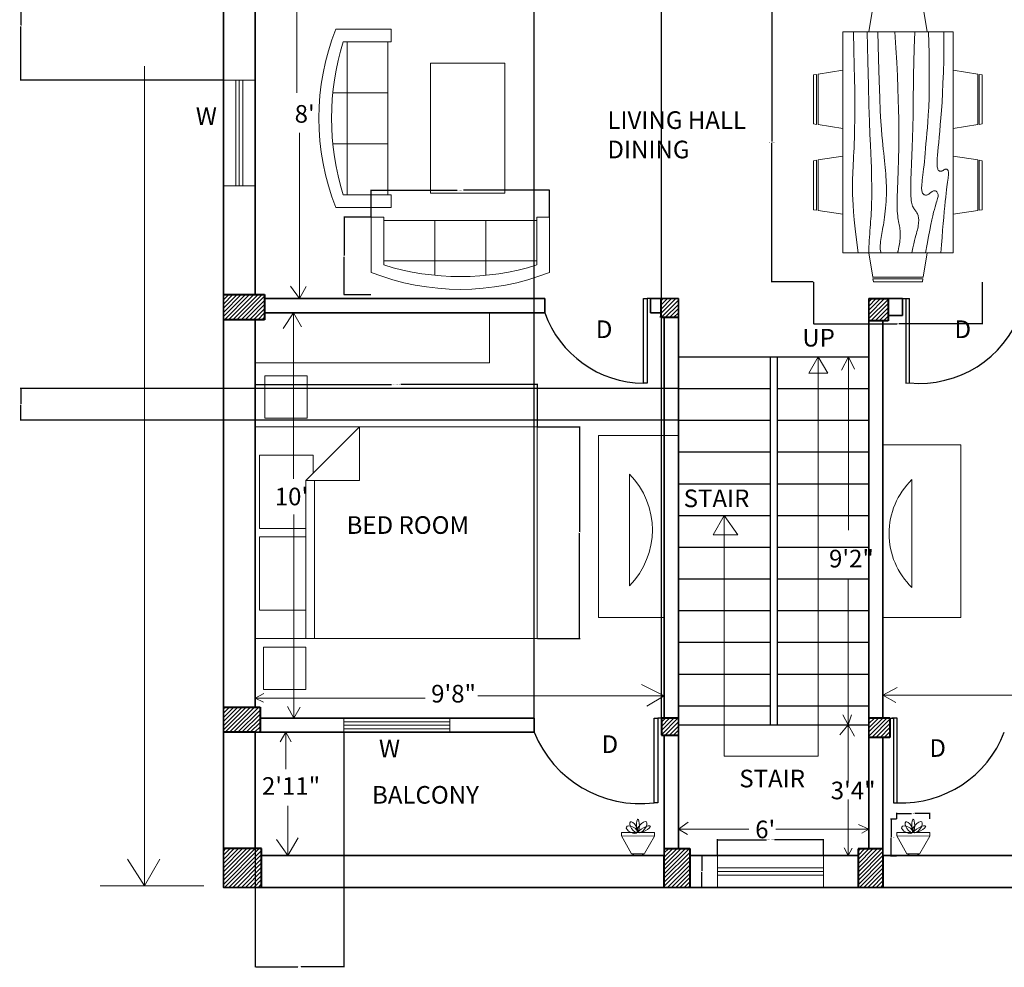
# Model space of a CAD drawing. Units: inches. Extents: x -34 to 385, y -422 to 64.
# Tile 1 of 3: x -34 to 246, y -422 to -153. Entities that reach past the tile are written whole.
import ezdxf

# ---------------------------------------------------------------- set-up
doc = ezdxf.new("R2010")
doc.units = ezdxf.units.IN
doc.header["$MEASUREMENT"] = 0
for name, color, linetype, lineweight in [('A-ANNO-DIMS', 2, 'Continuous', 13), ('A-ANNO-SYMB', 7, 'Continuous', 18), ('A-ANNO-TEXT', 7, 'Continuous', 18), ('A-AREA-IDEN', 7, 'Continuous', 25), ('A-COLS', 1, 'Continuous', 40), ('A-COLS-PATT', 252, 'Continuous', 13), ('A-DOOR', 3, 'Continuous', 25), ('A-FLOR-CASE', 32, 'Continuous', 20), ('A-FLOR-STRS', 7, 'Continuous', 25), ('A-FURN', 8, 'Continuous', 18), ('A-FURN-PLNT', 94, 'Continuous', 18), ('A-GLAZ', 4, 'Continuous', 18), ('A-WALL', 7, 'Continuous', 35)]:
    doc.layers.add(name, color=color, linetype=linetype, lineweight=lineweight)
doc.styles.get("Standard").update_dxf_attribs({"font": 'arial.ttf'})
doc.dimstyles.get("Standard").update_dxf_attribs({"dimtxt": 0.18, "dimasz": 0.18, "dimexe": 0.18, "dimexo": 0.0625, "dimgap": 0.09, "dimtad": 0, "dimtih": 1, "dimtoh": 1, "dimdec": 4, "dimzin": 0, "dimdsep": 46, "dimtxsty": 'Standard', "dimcen": 0.09, "dimadec": 0, "dimazin": 0, "dimtfac": 1, "dimtdec": 4, "dimtofl": 0, "dimtmove": 0, "dimatfit": 3, "dimfxl": 1, "dimtolj": 1, "dimtzin": 0, "dimarcsym": 0})

# ---------------------------------------------------------------- blocks, each defined once
blk = doc.blocks.new('Dining Set - 36 x 72 in.')
for p, q in [((-22.2343, 26.00059), (-23.4847, 17.99762)), ((-22.2304, 26), (-5.7608, 26)), ((-22, 27.5), (-22.1562, 26.50042)), ((-5.8416, 26.5), (-22.1534, 26.5)), ((-22, 27.5), (-6, 27.5)), ((-5.8437, 26.49966), (-6, 27.5)), ((-4.5152, 17.99762), (-5.7655, 25.99926)), ((5.7657, 26.00059), (4.5153, 17.99762)), ((5.7696, 26), (22.2392, 26)), ((6, 27.5), (5.8438, 26.50042)), ((22.1584, 26.5), (5.8466, 26.5)), ((6, 27.5), (22, 27.5)), ((22.1563, 26.49966), (22, 27.5)), ((23.4848, 17.99762), (22.2345, 25.99926)), ((36, 18), (-36, 18)), ((-36, 18), (-36, -18)), ((36, -18), (36, 18)), ((-45.5, 8), (-44.5004, 8.15617)), ((-45.5, 8), (-45.5, -8)), ((-44.5, -8.15843), (-44.5, 8.15338)), ((-44.0006, 8.23428), (-35.9976, 9.48474)), ((-44, 8.23041), (-44, -8.23915)), ((44.0006, 8.23428), (35.9976, 9.48474)), ((44, 8.23041), (44, -8.23915)), ((44.5, -8.15843), (44.5, 8.15338)), ((45.5, 8), (44.5005, 8.15617)), ((45.5, 8), (45.5, -8)), ((-44.4997, -8.15631), (-45.5, -8)), ((-35.9976, -9.48476), (-43.9993, -8.2345)), ((35.9976, -9.48476), (43.9993, -8.2345)), ((44.4997, -8.15631), (45.5, -8)), ((-36, -18), (36, -18)), ((-22.2343, -26.0006), (-23.4847, -17.99762)), ((-4.5152, -17.99762), (-5.7655, -25.99928)), ((5.7657, -26.0006), (4.5153, -17.99762)), ((23.4848, -17.99762), (22.2345, -25.99928)), ((-22.2304, -26), (-5.7608, -26)), ((-22, -27.5), (-22.1562, -26.50044)), ((-5.8416, -26.5), (-22.1534, -26.5)), ((-22, -27.5), (-6, -27.5)), ((-5.8437, -26.49967), (-6, -27.5)), ((5.7696, -26), (22.2392, -26)), ((6, -27.5), (5.8438, -26.50044)), ((22.1584, -26.5), (5.8466, -26.5)), ((6, -27.5), (22, -27.5)), ((22.1563, -26.49967), (22, -27.5))]:
    blk.add_line(p, q)
for points in [[(-36, 15), (-31.1772, 14.97754), (-26.8079, 14.91406), (-22.8538, 14.81543), (-19.276, 14.6875), (-16.0362, 14.53613), (-13.0957, 14.36718), (-10.4159, 14.18652), (-7.9583, 14), (-5.6904, 13.81315), (-3.6035, 13.63021), (-1.6954, 13.45508), (0.0365, 13.29166), (1.5945, 13.14388), (2.9811, 13.01562), (4.1988, 12.9108), (5.25, 12.83333), (6.1393, 12.78613), (6.8802, 12.76823), (7.4883, 12.77767), (7.9792, 12.8125), (8.3685, 12.87077), (8.6719, 12.95052), (8.9049, 13.0498), (9.0833, 13.16666), (9.2205, 13.29899), (9.3216, 13.44401), (9.3895, 13.59879), (9.4271, 13.76041), (9.4373, 13.92594), (9.4232, 14.09245), (9.3875, 14.257), (9.3333, 14.41666), (9.2638, 14.56917), (9.1836, 14.71484), (9.0975, 14.85465), (9.0104, 14.98958), (8.9272, 15.1206), (8.8529, 15.2487), (8.7922, 15.37483), (8.75, 15.5), (8.7305, 15.62467), (8.7344, 15.74739), (8.7617, 15.86621), (8.8125, 15.97916), (8.8867, 16.08431), (8.9844, 16.17968), (9.1055, 16.26334), (9.25, 16.33333), (9.4189, 16.38802), (9.6172, 16.42708), (9.8506, 16.45052), (10.125, 16.45833), (10.4463, 16.45052), (10.8203, 16.42708), (11.2529, 16.38802), (11.75, 16.33333), (12.3184, 16.26318), (12.9694, 16.17838), (13.7151, 16.07991), (14.5677, 15.96875), (15.5395, 15.84586), (16.6426, 15.71224), (17.8893, 15.56884), (19.2917, 15.41666), (20.859, 15.25667), (22.5879, 15.08984), (24.4721, 14.91715), (26.5052, 14.73958), (28.6809, 14.5581), (30.9929, 14.3737), (33.4347, 14.18733), (36, 14)], [(-36, 10), (-28.9766, 10.14274), (-23.1725, 10.20442), (-18.4241, 10.19775), (-14.5677, 10.13541), (-11.4399, 10.03011), (-8.877, 9.89453), (-6.7154, 9.74137), (-4.7917, 9.58333), (-2.9698, 9.43082), (-1.2246, 9.28515), (0.4415, 9.14534), (2.026, 9.01041), (3.5266, 8.87939), (4.9408, 8.7513), (6.266, 8.62516), (7.5, 8.5), (8.6411, 8.37549), (9.6914, 8.2539), (10.6538, 8.13818), (11.5312, 8.03125), (12.3267, 7.93603), (13.043, 7.85547), (13.6831, 7.79248), (14.25, 7.75), (14.7471, 7.7303), (15.1797, 7.73307), (15.5537, 7.75732), (15.875, 7.80208), (16.1494, 7.86637), (16.3828, 7.94922), (16.5811, 8.04964), (16.75, 8.16666), (16.8944, 8.29915), (17.0143, 8.44531), (17.1089, 8.60319), (17.1771, 8.77083), (17.218, 8.94629), (17.2305, 9.1276), (17.2137, 9.31282), (17.1667, 9.5), (17.0895, 9.6875), (16.987, 9.875), (16.8649, 10.0625), (16.7292, 10.25), (16.5856, 10.4375), (16.4401, 10.625), (16.2985, 10.8125), (16.1667, 11), (16.05, 11.18733), (15.9518, 11.3737), (15.8752, 11.5581), (15.8229, 11.73958), (15.798, 11.91715), (15.8034, 12.08984), (15.842, 12.25667), (15.9167, 12.41666), (16.0295, 12.56836), (16.1784, 12.70833), (16.3605, 12.83268), (16.5729, 12.9375), (16.8127, 13.01888), (17.0768, 13.07291), (17.3625, 13.0957), (17.6667, 13.08333), (17.9894, 13.03312), (18.3418, 12.94726), (18.7382, 12.82918), (19.1927, 12.68229), (19.7195, 12.51001), (20.3327, 12.31575), (21.0465, 12.10294), (21.875, 11.875), (22.8357, 11.63354), (23.959, 11.37304), (25.2786, 11.08618), (26.8282, 10.76562), (28.6414, 10.40405), (30.752, 9.99414), (33.1936, 9.52856), (36, 9)], [(-36, 5.5), (-30.7157, 5.3348), (-26.069, 5.20963), (-21.9946, 5.11767), (-18.4271, 5.05208), (-15.3009, 5.00602), (-12.5508, 4.97265), (-10.1112, 4.94515), (-7.9167, 4.91666), (-5.909, 4.88167), (-4.0586, 4.83984), (-2.3429, 4.79215), (-0.7396, 4.73958), (0.7739, 4.6831), (2.22, 4.6237), (3.6213, 4.56233), (5, 4.5), (6.373, 4.43782), (7.7344, 4.3776), (9.0723, 4.32129), (10.375, 4.27083), (11.6309, 4.22819), (12.8281, 4.19531), (13.9551, 4.17415), (15, 4.16666), (15.954, 4.17448), (16.819, 4.19791), (17.6001, 4.23698), (18.3021, 4.29166), (18.9299, 4.36198), (19.4883, 4.44791), (19.9823, 4.54948), (20.4167, 4.66666), (20.7969, 4.79899), (21.1302, 4.94401), (21.4245, 5.09879), (21.6875, 5.26041), (21.9271, 5.42594), (22.1511, 5.59245), (22.3672, 5.757), (22.5834, 5.91666), (22.8065, 6.06868), (23.0404, 6.21093), (23.2879, 6.34147), (23.5521, 6.45833), (23.8358, 6.55957), (24.142, 6.64323), (24.4735, 6.70735), (24.8334, 6.75), (25.2235, 6.76969), (25.642, 6.76692), (26.0858, 6.74267), (26.5521, 6.69791), (27.0379, 6.63362), (27.5404, 6.55078), (28.0565, 6.45036), (28.5834, 6.33333), (29.1242, 6.19987), (29.7071, 6.04687), (30.3661, 5.87044), (31.1354, 5.66666), (32.0493, 5.43164), (33.142, 5.16146), (34.4475, 4.85221), (36, 4.5)], [(-36, -1), (-30.7915, -0.6591), (-26.0195, -0.38216), (-21.6519, -0.16284), (-17.6563, 0.00521), (-14.0005, 0.12833), (-10.6523, 0.21289), (-7.5796, 0.26522), (-4.75, 0.29166), (-2.134, 0.29793), (0.2878, 0.28711), (2.5317, 0.26163), (4.6146, 0.22396), (6.5529, 0.17651), (8.3633, 0.12174), (10.0623, 0.06209), (11.6667, 0), (13.1899, -0.06201), (14.6341, -0.1211), (15.9982, -0.17432), (17.2813, -0.21875), (18.4823, -0.25147), (19.6003, -0.26953), (20.6343, -0.27002), (21.5834, -0.25), (22.4481, -0.20768), (23.2357, -0.14584), (23.9549, -0.06836), (24.6146, 0.02083), (25.2235, 0.11784), (25.7904, 0.21875), (26.3241, 0.31966), (26.8334, 0.41666), (27.3265, 0.50618), (27.8099, 0.58593), (28.2894, 0.65397), (28.7709, 0.70833), (29.2601, 0.74707), (29.763, 0.76823), (30.2855, 0.76985), (30.8334, 0.75), (31.4088, 0.70784), (31.9994, 0.64713), (32.589, 0.57275), (33.1615, 0.48958), (33.7008, 0.4025), (34.1908, 0.3164), (34.6153, 0.23616), (34.9584, 0.16666), (35.2099, 0.11165), (35.3848, 0.07031), (35.504, 0.04069), (35.5886, 0.02083), (35.6594, 0.00879), (35.7377, 0.0026), (35.8442, 0.00032), (36, 0)], [(-36, -6.5), (-27.1843, -6.31267), (-20.084, -6.1263), (-14.469, -5.9419), (-10.1094, -5.76042), (-6.7752, -5.58285), (-4.2363, -5.41016), (-2.2629, -5.24333), (-0.625, -5.08334), (0.8708, -4.93099), (2.2715, -4.78646), (3.5872, -4.64974), (4.8281, -4.52084), (6.0046, -4.39974), (7.127, -4.28646), (8.2053, -4.18099), (9.25, -4.08334), (10.2705, -3.99382), (11.2734, -3.91407), (12.2647, -3.84603), (13.25, -3.79167), (14.2354, -3.75293), (15.2266, -3.73177), (16.2295, -3.73015), (17.25, -3.75), (18.2912, -3.79248), (19.3451, -3.85547), (20.4009, -3.93604), (21.4479, -4.03125), (22.4754, -4.13819), (23.4727, -4.25391), (24.4289, -4.37549), (25.3334, -4.5), (26.1785, -4.62492), (26.9694, -4.74935), (27.7145, -4.87281), (28.4219, -4.99479), (29.1, -5.11483), (29.7572, -5.23242), (30.4016, -5.34709), (31.0417, -5.45834), (31.6837, -5.56437), (32.3262, -5.65821), (32.9658, -5.73153), (33.599, -5.77604), (34.2224, -5.78345), (34.8327, -5.74545), (35.4264, -5.65373), (36, -5.5)], [(-36, -10), (-26.4022, -9.81299), (-18.4675, -9.62891), (-11.9839, -9.45069), (-6.7396, -9.28125), (-2.5226, -9.12354), (0.8789, -8.98047), (3.6769, -8.85498), (6.0833, -8.75), (8.2767, -8.66765), (10.3021, -8.60677), (12.1712, -8.56543), (13.8958, -8.54167), (15.4876, -8.53353), (16.9583, -8.53907), (18.3197, -8.55632), (19.5834, -8.58334), (20.7616, -8.61841), (21.8685, -8.66081), (22.9188, -8.71004), (23.9271, -8.76563), (24.9081, -8.82707), (25.8763, -8.89388), (26.8465, -8.96558), (27.8334, -9.04167), (28.8474, -9.12118), (29.8828, -9.20117), (30.93, -9.27824), (31.9792, -9.34896), (33.0205, -9.40991), (34.0443, -9.45768), (35.0407, -9.48885), (36, -9.5)], [(-36, -14.5), (-30.0881, -14.33513), (-25.0332, -14.21224), (-20.7312, -14.12647), (-17.0781, -14.07292), (-13.97, -14.04671), (-11.3027, -14.04297), (-8.9724, -14.05681), (-6.875, -14.08334), (-4.9224, -14.11833), (-3.0905, -14.16016), (-1.3709, -14.20785), (0.2448, -14.26042), (1.7647, -14.3169), (3.1973, -14.3763), (4.5507, -14.43767), (5.8333, -14.5), (7.0554, -14.5621), (8.235, -14.62175), (9.3922, -14.67652), (10.5469, -14.72396), (11.7192, -14.76164), (12.929, -14.78711), (14.1965, -14.79794), (15.5417, -14.79167), (16.9933, -14.76424), (18.6152, -14.70508), (20.4804, -14.60197), (22.6615, -14.44271), (25.2312, -14.21509), (28.2624, -13.9069), (31.8277, -13.50594), (36, -13)]]:
    blk.add_lwpolyline(points)
blk = doc.blocks.new('Sofa - Roundback 7 ft.')
for p, q in [((-12.00002, -32.4421), (-12.00003, -6.5971)), ((11.99997, -32.4421), (11.99998, -6.5971)), ((-36.000027, -34), (-36.000027, -11.4696)), ((-35.999844, -13.3819), (35.9998, -13.3819)), ((35.99998, -34), (35.99998, -11.4696)), ((-36.000027, -32.4421), (35.99998, -32.4421))]:
    blk.add_line(p, q)
for points in [[(-36.000027, -34), (-42.000027, -34), (-42.000027, -8)], [(41.99998, -8), (41.99998, -34), (35.99998, -34)]]:
    blk.add_lwpolyline(points)
for centre, radius, start, end in [((0, -114.25), 114.25, 68.43141, 111.5686), ((-0.00001, -127.1968), 121.1968, 72.72033, 107.2797)]:
    blk.add_arc(centre, radius, start, end)
blk = doc.blocks.new('Bed - Queen')
for p, q in [((0, -80.00003), (0, 0)), ((0, 0), (59.99999, 0)), ((59.99999, 0), (59.99999, -80.00003)), ((7.99999, -1.2), (28.79998, -1.2)), ((7.99999, -14.4), (7.99999, -1.2)), ((28.79998, -1.2), (28.79998, -14.4)), ((31.19999, -1.2), (51.99999, -1.2)), ((31.19999, -14.4), (31.19999, -1.2)), ((51.99999, -1.2), (51.99999, -16.4)), ((0, -14.4), (44.8, -14.4)), ((59.99999, -29.6), (44.8, -14.4)), ((44.8, -14.4), (44.8, -29.6)), ((51.99999, -16.4), (46.79936, -16.4)), ((44.8, -16.8), (0, -16.8)), ((44.8, -29.6), (59.99999, -29.6)), ((59.99999, -80.00003), (0, -80.00003))]:
    blk.add_line(p, q)
blk = doc.blocks.new('WIN-30IN-9IN-WALL')
for p, q in [((0, 9), (0, 0)), ((30, 9), (30, 0)), ((0, 5.5), (30, 5.5)), ((0, 4.5), (30, 4.5)), ((0, 3.5), (30, 3.5))]:
    blk.add_line(p, q)
blk = doc.blocks.new('WIN-30IN-4IN-WALL')
for p, q in [((0, 4), (0, 0)), ((0, 3), (30, 3)), ((30, 4), (30, 0)), ((0, 2), (30, 2)), ((0, 1), (30, 1))]:
    blk.add_line(p, q)
blk = doc.blocks.new('DOOR-LEAF-24IN')
for p, q in [((1, 24), (0, 24)), ((0, 24), (0, 0)), ((1, 0), (1, 24)), ((0, 0), (1, 0)), ((2, 0), (1, 0))]:
    blk.add_line(p, q)
blk = doc.blocks.new('NIGHTSTAND-12IN')
blk.add_lwpolyline([(12, 0), (0, 0), (0, 12), (12, 12)], close=True)
blk = doc.blocks.new('BALCONY-PLANTER')
for p, q in [((0, 5.57), (0, 6.56)), ((0, 6.56), (9.42, 6.56)), ((9.42, 6.56), (9.42, 5.54)), ((2.92, 0.52), (0, 5.57)), ((0, 5.57), (9.42, 5.54)), ((9.42, 5.54), (6.54, 0.56))]:
    blk.add_line(p, q)
blk.add_arc((4.7, 3.31), 3.31, 237.326, 303.729)
for centre, major_axis, ratio in [((2.96, 7.36), (1.54, -0.75), 0.479353), ((3.53, 8.09), (0.98, -1.48), 0.414718), ((4.71, 8.47), (0, -1.91), 0.211909), ((5.9, 8.07), (-1.19, -1.51), 0.459362), ((6.52, 7.49), (-1.74, -0.91), 0.246731)]:
    blk.add_ellipse(centre, major_axis=major_axis, ratio=ratio)
blk = doc.blocks.new('*D14')
at = {"layer": 'A-ANNO-DIMS', "color": 0, "lineweight": -2, "transparency": 16777216}
for p, q in [((164.36, -390.08), (164.36, -385.46)), ((164.54, -385.64), (178.24, -385.64)), ((194.18, -385.64), (180.48, -385.64)), ((194.36, -390.08), (194.36, -385.46))]:
    blk.add_line(p, q, dxfattribs=at)
at = {"layer": 'A-ANNO-DIMS', "color": 0, "transparency": 16777216}
for points in [[(164.54, -385.61), (164.54, -385.67), (164.36, -385.64)], [(194.18, -385.61), (194.18, -385.67), (194.36, -385.64)]]:
    blk.add_solid(points, dxfattribs=at)
at = {"layer": 'Defpoints', "color": 0, "transparency": 16777216}
for p in [(194.36, -385.64), (164.36, -390.14), (194.36, -390.14)]:
    blk.add_point(p, dxfattribs=at)
at = {"layer": 'A-ANNO-DIMS', "color": 0, "transparency": 16777216, "insert": (179.36, -385.64), "char_height": 0.18, "attachment_point": 5}
blk.add_mtext('\\A1;WINDOW 30 TYP.', dxfattribs=at)
blk = doc.blocks.new('*D15')
at = {"layer": 'A-ANNO-DIMS', "color": 0, "lineweight": -2, "transparency": 16777216}
for p, q in [((164.3, -390.14), (159.68, -390.14)), ((159.86, -390.32), (159.86, -394.46)), ((159.86, -398.96), (159.86, -394.82)), ((164.3, -399.14), (159.68, -399.14))]:
    blk.add_line(p, q, dxfattribs=at)
at = {"layer": 'A-ANNO-DIMS', "color": 0, "transparency": 16777216}
for points in [[(159.83, -390.32), (159.89, -390.32), (159.86, -390.14)], [(159.83, -398.96), (159.89, -398.96), (159.86, -399.14)]]:
    blk.add_solid(points, dxfattribs=at)
at = {"layer": 'Defpoints', "color": 0, "transparency": 16777216}
for p in [(159.86, -390.14), (164.36, -390.14), (164.36, -399.14)]:
    blk.add_point(p, dxfattribs=at)
at = {"layer": 'A-ANNO-DIMS', "color": 0, "transparency": 16777216, "insert": (159.86, -394.64), "char_height": 0.18, "attachment_point": 5}
blk.add_mtext('\\A1;9 TYP.', dxfattribs=at)
blk = doc.blocks.new('*D20')
at = {"layer": 'A-ANNO-DIMS', "color": 0, "lineweight": -2, "transparency": 16777216}
for p, q in [((33.26, -268.45), (33.26, -256.33)), ((33.44, -256.51), (71.95, -256.51)), ((113.08, -256.51), (74.56, -256.51)), ((113.26, -268.45), (113.26, -256.33))]:
    blk.add_line(p, q, dxfattribs=at)
at = {"layer": 'A-ANNO-DIMS', "color": 0, "transparency": 16777216}
for points in [[(33.44, -256.48), (33.44, -256.54), (33.26, -256.51)], [(113.08, -256.48), (113.08, -256.54), (113.26, -256.51)]]:
    blk.add_solid(points, dxfattribs=at)
at = {"layer": 'Defpoints', "color": 0, "transparency": 16777216}
for p in [(33.26, -256.51), (33.26, -268.51), (113.26, -268.51)]:
    blk.add_point(p, dxfattribs=at)
at = {"layer": 'A-ANNO-DIMS', "color": 0, "transparency": 16777216, "insert": (73.26, -256.51), "char_height": 0.18, "attachment_point": 5}
blk.add_mtext('\\A1;QUEEN BED 80 TYP.', dxfattribs=at)
blk = doc.blocks.new('*D21')
at = {"layer": 'A-ANNO-DIMS', "color": 0, "lineweight": -2, "transparency": 16777216}
for p, q in [((113.32, -268.51), (125.44, -268.51)), ((125.26, -268.69), (125.26, -298.33)), ((125.26, -328.33), (125.26, -298.7)), ((113.32, -328.51), (125.44, -328.51))]:
    blk.add_line(p, q, dxfattribs=at)
at = {"layer": 'A-ANNO-DIMS', "color": 0, "transparency": 16777216}
for points in [[(125.23, -268.69), (125.29, -268.69), (125.26, -268.51)], [(125.23, -328.33), (125.29, -328.33), (125.26, -328.51)]]:
    blk.add_solid(points, dxfattribs=at)
at = {"layer": 'Defpoints', "color": 0, "transparency": 16777216}
for p in [(113.26, -268.51), (125.26, -268.51), (113.26, -328.51)]:
    blk.add_point(p, dxfattribs=at)
at = {"layer": 'A-ANNO-DIMS', "color": 0, "transparency": 16777216, "insert": (125.26, -298.51), "char_height": 0.18, "attachment_point": 5}
blk.add_mtext('\\A1;60 TYP.', dxfattribs=at)
blk = doc.blocks.new('*D22')
at = {"layer": 'A-ANNO-DIMS', "color": 0, "lineweight": -2, "transparency": 16777216}
for p, q in [((66.13, -208.95), (66.13, -201.24)), ((66.31, -201.42), (90.53, -201.42)), ((116.57, -201.42), (92.34, -201.42)), ((116.75, -208.95), (116.75, -201.24))]:
    blk.add_line(p, q, dxfattribs=at)
at = {"layer": 'A-ANNO-DIMS', "color": 0, "transparency": 16777216}
for points in [[(66.31, -201.39), (66.31, -201.45), (66.13, -201.42)], [(116.57, -201.39), (116.57, -201.45), (116.75, -201.42)]]:
    blk.add_solid(points, dxfattribs=at)
at = {"layer": 'Defpoints', "color": 0, "transparency": 16777216}
for p in [(66.13, -201.42), (66.13, -209.01), (116.75, -209.01)]:
    blk.add_point(p, dxfattribs=at)
at = {"layer": 'A-ANNO-DIMS', "color": 0, "transparency": 16777216, "insert": (91.44, -201.42), "char_height": 0.18, "attachment_point": 5}
blk.add_mtext('\\A1;SOFA 51 TYP.', dxfattribs=at)
blk = doc.blocks.new('*D23')
at = {"layer": 'A-ANNO-DIMS', "color": 0, "lineweight": -2, "transparency": 16777216}
for p, q in [((66.06, -209.01), (58.35, -209.01)), ((58.53, -209.19), (58.53, -219.88)), ((58.53, -230.93), (58.53, -220.24)), ((66.06, -231.11), (58.35, -231.11))]:
    blk.add_line(p, q, dxfattribs=at)
at = {"layer": 'A-ANNO-DIMS', "color": 0, "transparency": 16777216}
for points in [[(58.5, -209.19), (58.56, -209.19), (58.53, -209.01)], [(58.5, -230.93), (58.56, -230.93), (58.53, -231.11)]]:
    blk.add_solid(points, dxfattribs=at)
at = {"layer": 'Defpoints', "color": 0, "transparency": 16777216}
for p in [(66.13, -209.01), (58.53, -231.11), (66.13, -231.11)]:
    blk.add_point(p, dxfattribs=at)
at = {"layer": 'A-ANNO-DIMS', "color": 0, "transparency": 16777216, "insert": (58.53, -220.06), "char_height": 0.18, "attachment_point": 5}
blk.add_mtext('\\A1;22 TYP.', dxfattribs=at)
blk = doc.blocks.new('*D26')
at = {"layer": 'A-ANNO-DIMS', "color": 0, "lineweight": -2, "transparency": 16777216}
for p, q in [((215.08, -379.77), (213.38, -379.77)), ((213.56, -379.95), (213.56, -384.87)), ((213.56, -390.15), (213.56, -385.23)), ((215.08, -390.33), (213.38, -390.33))]:
    blk.add_line(p, q, dxfattribs=at)
at = {"layer": 'A-ANNO-DIMS', "color": 0, "transparency": 16777216}
for points in [[(213.53, -379.95), (213.59, -379.95), (213.56, -379.77)], [(213.53, -390.15), (213.59, -390.15), (213.56, -390.33)]]:
    blk.add_solid(points, dxfattribs=at)
at = {"layer": 'Defpoints', "color": 0, "transparency": 16777216}
for p in [(213.56, -379.77), (215.14, -379.77), (215.14, -390.33)]:
    blk.add_point(p, dxfattribs=at)
at = {"layer": 'A-ANNO-DIMS', "color": 0, "transparency": 16777216, "insert": (213.56, -385.05), "char_height": 0.18, "attachment_point": 5}
blk.add_mtext('\\A1;PLANTER 11 TYP.', dxfattribs=at)
blk = doc.blocks.new('*D27')
at = {"layer": 'A-ANNO-DIMS', "color": 0, "lineweight": -2, "transparency": 16777216}
for p, q in [((215.14, -379.7), (215.14, -378)), ((215.32, -378.18), (219.39, -378.18)), ((224.38, -378.18), (220.31, -378.18)), ((224.56, -379.7), (224.56, -378))]:
    blk.add_line(p, q, dxfattribs=at)
at = {"layer": 'A-ANNO-DIMS', "color": 0, "transparency": 16777216}
for points in [[(215.32, -378.15), (215.32, -378.21), (215.14, -378.18)], [(224.38, -378.15), (224.38, -378.21), (224.56, -378.18)]]:
    blk.add_solid(points, dxfattribs=at)
at = {"layer": 'Defpoints', "color": 0, "transparency": 16777216}
for p in [(224.56, -378.18), (215.14, -379.77), (224.56, -379.77)]:
    blk.add_point(p, dxfattribs=at)
at = {"layer": 'A-ANNO-DIMS', "color": 0, "transparency": 16777216, "insert": (219.85, -378.18), "char_height": 0.18, "attachment_point": 5}
blk.add_mtext('\\A1;9 TYP.', dxfattribs=at)
blk = doc.blocks.new('*D32')
at = {"layer": 'A-ANNO-DIMS', "color": 0, "lineweight": -2, "transparency": 16777216}
for p, q in [((191.51, -148.21), (179.52, -148.21)), ((179.7, -148.39), (179.7, -187.61)), ((179.7, -227.2), (179.7, -187.98)), ((191.51, -227.38), (179.52, -227.38))]:
    blk.add_line(p, q, dxfattribs=at)
at = {"layer": 'A-ANNO-DIMS', "color": 0, "transparency": 16777216}
for points in [[(179.67, -148.39), (179.73, -148.39), (179.7, -148.21)], [(179.67, -227.2), (179.73, -227.2), (179.7, -227.38)]]:
    blk.add_solid(points, dxfattribs=at)
at = {"layer": 'Defpoints', "color": 0, "transparency": 16777216}
for p in [(191.58, -148.21), (179.7, -227.38), (191.58, -227.38)]:
    blk.add_point(p, dxfattribs=at)
at = {"layer": 'A-ANNO-DIMS', "color": 0, "transparency": 16777216, "insert": (179.7, -187.79), "char_height": 0.18, "attachment_point": 5}
blk.add_mtext('\\A1;DINING SET 79', dxfattribs=at)
blk = doc.blocks.new('*D33')
at = {"layer": 'A-ANNO-DIMS', "color": 0, "lineweight": -2, "transparency": 16777216}
for p, q in [((191.58, -227.44), (191.58, -239.43)), ((239.42, -227.44), (239.42, -239.43)), ((191.76, -239.25), (215.28, -239.25)), ((239.24, -239.25), (215.72, -239.25))]:
    blk.add_line(p, q, dxfattribs=at)
at = {"layer": 'A-ANNO-DIMS', "color": 0, "transparency": 16777216}
for points in [[(191.76, -239.22), (191.76, -239.28), (191.58, -239.25)], [(239.24, -239.22), (239.24, -239.28), (239.42, -239.25)]]:
    blk.add_solid(points, dxfattribs=at)
at = {"layer": 'Defpoints', "color": 0, "transparency": 16777216}
for p in [(191.58, -227.38), (239.42, -227.38), (239.42, -239.25)]:
    blk.add_point(p, dxfattribs=at)
at = {"layer": 'A-ANNO-DIMS', "color": 0, "transparency": 16777216, "insert": (215.5, -239.25), "char_height": 0.18, "attachment_point": 5}
blk.add_mtext('\\A1;48', dxfattribs=at)
blk = doc.blocks.new('*D36')
at = {"layer": 'A-ANNO-DIMS', "color": 0, "lineweight": -2, "transparency": 16777216}
for p, q in [((24.19, -139.38), (-33.38, -139.38)), ((-33.2, -139.56), (-33.2, -154.58)), ((-33.2, -169.95), (-33.2, -154.94)), ((24.19, -170.13), (-33.38, -170.13))]:
    blk.add_line(p, q, dxfattribs=at)
at = {"layer": 'A-ANNO-DIMS', "color": 0, "transparency": 16777216}
for points in [[(-33.23, -139.56), (-33.17, -139.56), (-33.2, -139.38)], [(-33.23, -169.95), (-33.17, -169.95), (-33.2, -170.13)]]:
    blk.add_solid(points, dxfattribs=at)
at = {"layer": 'Defpoints', "color": 0, "transparency": 16777216}
for p in [(24.26, -139.38), (-33.2, -170.13), (24.26, -170.13)]:
    blk.add_point(p, dxfattribs=at)
at = {"layer": 'A-ANNO-DIMS', "color": 0, "transparency": 16777216, "insert": (-33.2, -154.76), "char_height": 0.18, "attachment_point": 5}
blk.add_mtext('\\A1;30.75', dxfattribs=at)
blk = doc.blocks.new('*D38')
at = {"layer": 'A-ANNO-DIMS', "color": 0, "lineweight": -2, "transparency": 16777216}
for p, q in [((153.19, -257.63), (-33.38, -257.63)), ((-33.2, -257.81), (-33.2, -261.95)), ((-33.2, -266.45), (-33.2, -262.31)), ((153.19, -266.63), (-33.38, -266.63))]:
    blk.add_line(p, q, dxfattribs=at)
at = {"layer": 'A-ANNO-DIMS', "color": 0, "transparency": 16777216}
for points in [[(-33.23, -257.81), (-33.17, -257.81), (-33.2, -257.63)], [(-33.23, -266.45), (-33.17, -266.45), (-33.2, -266.63)]]:
    blk.add_solid(points, dxfattribs=at)
at = {"layer": 'Defpoints', "color": 0, "transparency": 16777216}
for p in [(153.26, -257.63), (-33.2, -266.63), (153.26, -266.63)]:
    blk.add_point(p, dxfattribs=at)
at = {"layer": 'A-ANNO-DIMS', "color": 0, "transparency": 16777216, "insert": (-33.2, -262.13), "char_height": 0.18, "attachment_point": 5}
blk.add_mtext('\\A1;9', dxfattribs=at)
blk = doc.blocks.new('*D39')
at = {"layer": 'A-ANNO-DIMS', "color": 0, "lineweight": -2, "transparency": 16777216}
for p, q in [((112.34, -351.08), (112.34, 63.89)), ((112.52, 63.71), (129.99, 63.71)), ((148.25, 63.71), (130.78, 63.71)), ((148.43, -351.08), (148.43, 63.89))]:
    blk.add_line(p, q, dxfattribs=at)
at = {"layer": 'A-ANNO-DIMS', "color": 0, "transparency": 16777216}
for points in [[(112.52, 63.74), (112.52, 63.68), (112.34, 63.71)], [(148.25, 63.74), (148.25, 63.68), (148.43, 63.71)]]:
    blk.add_solid(points, dxfattribs=at)
at = {"layer": 'Defpoints', "color": 0, "transparency": 16777216}
for p in [(148.43, 63.71), (112.34, -351.14), (148.43, -351.14)]:
    blk.add_point(p, dxfattribs=at)
at = {"layer": 'A-ANNO-DIMS', "color": 0, "transparency": 16777216, "insert": (130.38, 63.71), "char_height": 0.18, "attachment_point": 5}
blk.add_mtext('\\A1;36.09', dxfattribs=at)
blk = doc.blocks.new('*D40')
at = {"layer": 'A-ANNO-DIMS', "color": 0, "lineweight": -2, "transparency": 16777216}
for p, q in [((33.26, -355.21), (33.26, -421.82)), ((58.42, -355.21), (58.42, -421.82)), ((33.44, -421.64), (45.37, -421.64)), ((58.24, -421.64), (46.3, -421.64))]:
    blk.add_line(p, q, dxfattribs=at)
at = {"layer": 'A-ANNO-DIMS', "color": 0, "transparency": 16777216}
for points in [[(33.44, -421.61), (33.44, -421.67), (33.26, -421.64)], [(58.24, -421.61), (58.24, -421.67), (58.42, -421.64)]]:
    blk.add_solid(points, dxfattribs=at)
at = {"layer": 'Defpoints', "color": 0, "transparency": 16777216}
for p in [(33.26, -355.14), (58.42, -355.14), (58.42, -421.64)]:
    blk.add_point(p, dxfattribs=at)
at = {"layer": 'A-ANNO-DIMS', "color": 0, "transparency": 16777216, "insert": (45.84, -421.64), "char_height": 0.18, "attachment_point": 5}
blk.add_mtext('\\A1;25.166', dxfattribs=at)

msp = doc.modelspace()

# ---------------------------------------------------------------- hatches: boundary and pattern name
at = {"layer": 'A-COLS-PATT'}
h = msp.add_hatch(dxfattribs=at)
h.set_pattern_fill('ANSI31', color=256, scale=6.7)
h.set_pattern_definition([(45, (-1587.6103, -800.894), (-0.59220193, 0.59220193), [])])
h.paths.add_polyline_path([(34.5325, 20.857), (24.2567, 20.857), (24.2567, 10.5552), (34.5325, 10.5552)])
h.paths.add_polyline_path([(155.6882, 20.857), (147.6505, 20.857), (147.6505, 8.8355), (155.6882, 8.8355)])
h.paths.add_polyline_path([(214.1102, 20.857), (204.3358, 20.857), (204.3358, 9.8804), (214.1102, 9.8804)])
h.paths.add_polyline_path([(336.2567, 20.857), (324.9664, 20.857), (324.9664, 9.4113), (336.2567, 9.4113)])
h.paths.add_polyline_path([(336.2567, -129.6656), (324.4892, -129.6656), (324.4892, -138.8931), (336.2567, -138.8931)])
h.paths.add_polyline_path([(212.9763, -130.7216), (204.8831, -130.7216), (204.8831, -136.143), (212.9763, -136.143)])
h.paths.add_polyline_path([(154.6774, -130.7571), (147.9004, -130.7571), (147.9004, -136.143), (154.6774, -136.143)])
h.paths.add_polyline_path([(36.3503, -129.7825), (24.2567, -129.7825), (24.2567, -139.3836), (36.3503, -139.3836)])
h.paths.add_polyline_path([(35.9496, -230.9729), (24.2567, -230.9729), (24.2567, -238.1404), (35.9496, -238.1404)])
h.paths.add_polyline_path([(153.2567, -232.143), (148.2796, -232.143), (148.2796, -237.1221), (148.2796, -237.5145), (153.2567, -237.5145)])
h.paths.add_polyline_path([(212.7, -232.143), (207.2567, -232.143), (207.2567, -238.4312), (212.7, -238.4312)])
h.paths.add_polyline_path([(336.2567, -230.9985), (325.0216, -230.9985), (325.0216, -236.8618), (336.2567, -236.8618)])
h.paths.add_polyline_path([(34.6412, -348.0183), (24.2567, -348.0183), (24.2567, -355.143), (33.2567, -355.143), (34.6412, -355.143)])
h.paths.add_polyline_path([(35.0834, -388.1327), (24.2567, -388.1327), (24.2567, -399.143), (35.0834, -399.143)])
h.paths.add_polyline_path([(156.485, -388.1078), (149.2567, -388.1078), (149.2567, -390.143), (149.2567, -399.143), (156.485, -399.143)])
h.paths.add_polyline_path([(153.2567, -351.143), (148.4284, -351.143), (148.4284, -355.9617), (153.2567, -355.9617)])
h.paths.add_polyline_path([(211.2567, -390.143), (211.2567, -388.2391), (204.1967, -388.2391), (204.1967, -399.143), (211.2567, -399.143)])
h.paths.add_polyline_path([(213.2403, -351.143), (207.2567, -351.143), (207.2567, -356.6203), (213.2403, -356.6203)])
h.paths.add_polyline_path([(336.2567, -347.847), (325.718, -347.847), (325.718, -355.143), (327.2567, -355.143), (336.2567, -355.143)])
h.paths.add_polyline_path([(336.2567, -387.9228), (324.3995, -387.9228), (324.3995, -399.143), (336.2567, -399.143)])

# ---------------------------------------------------------------- linework, layer by layer
at = {"layer": 'A-ANNO-DIMS'}
for p, q in [((45.0444, -136.143), (45.0444, -173.7502)), ((1.8374, -166.2149), (1.8374, -398.7115)), ((45.78, -185.1463), (45.78, -232.143)), ((43.3216, -228.5632), (45.78, -232.143)), ((45.78, -232.143), (47.7571, -228.7186)), ((41.1963, -240.6314), (44.1164, -236.143)), ((44.1164, -236.143), (44.1164, -283.2275)), ((44.1164, -236.143), (46.4329, -240.1553)), ((199.4983, -252.4039), (201.493, -248.6296)), ((201.493, -297.8599), (201.493, -248.6296)), ((201.493, -248.6296), (203.2313, -252.1189)), ((44.2385, -293.3445), (44.2385, -351.143)), ((201.3501, -353.0127), (201.3501, -311.6296)), ((142.7633, -341.59), (149.2567, -344.8428)), ((215.2751, -342.4236), (211.2567, -344.6286)), ((35.7441, -344.1959), (33.2567, -345.4703)), ((81.4852, -345.4703), (33.2567, -345.4703)), ((33.2567, -345.4703), (35.6109, -346.6262)), ((96.4189, -344.8428), (149.2567, -344.8428)), ((149.2567, -344.8428), (144.2823, -347.7148)), ((211.2567, -344.6286), (263.9083, -344.6286)), ((211.2567, -344.6286), (214.8687, -346.714)), ((42.4108, -347.8273), (44.2385, -351.143)), ((44.2385, -351.143), (46.0452, -348.0137)), ((199.8513, -350.1619), (201.3501, -353.0127)), ((201.3501, -353.0127), (202.3704, -350.2199)), ((199.0262, -355.8552), (201.3501, -353.0127)), ((201.3501, -353.0127), (201.3501, -369.1556)), ((201.3501, -353.0127), (203.231, -356.2705)), ((40.32, -357.8461), (41.9326, -355.143)), ((41.9326, -365.6065), (41.9326, -355.143)), ((41.9326, -355.143), (43.4761, -357.8165)), ((42.5556, -376.0325), (42.5556, -390.143)), ((201.3505, -390.143), (201.3505, -374.2647)), ((156.0162, -380.6879), (153.2567, -382.6453)), ((204.2931, -381.3085), (207.2567, -382.5976)), ((42.5556, -390.143), (45.478, -385.0813)), ((153.2567, -382.6453), (173.2716, -382.6453)), ((153.2567, -382.6453), (155.8803, -384.1601)), ((180.8716, -382.5976), (207.2567, -382.5976)), ((207.2567, -382.5976), (205.2342, -383.7653)), ((39.3061, -385.5198), (42.5556, -390.143)), ((200.2241, -387.9357), (201.3505, -390.143)), ((201.3505, -390.143), (202.5556, -388.0557)), ((-2.9226, -391.1375), (1.8374, -398.7115)), ((1.8374, -398.7115), (6.1985, -391.1579)), ((-5.3558, -398.7115), (-10.6993, -398.7115)), ((18.7263, -398.7115), (-5.3558, -398.7115))]:
    msp.add_line(p, q, dxfattribs=at)
at = {"layer": 'A-ANNO-SYMB'}
for p, q in [((190.2026, -253.2734), (192.9072, -248.6296)), ((192.9072, -248.6296), (192.9072, -361.8808)), ((192.9072, -248.6296), (195.5804, -253.2596)), ((195.5804, -253.2596), (190.2106, -253.2596)), ((166.2567, -293.6296), (163.0736, -299.1428)), ((166.2567, -293.6296), (166.2567, -361.8808)), ((170.1172, -299.1428), (166.2567, -293.6296)), ((163.0736, -299.1428), (170.1172, -299.1428)), ((192.9072, -361.8808), (166.2567, -361.8808))]:
    msp.add_line(p, q, dxfattribs=at)
at = {"layer": 'A-COLS'}
for p, q in [((24.2567, -230.9729), (35.9496, -230.9729)), ((35.9496, -230.9729), (35.9496, -238.1404)), ((148.2796, -232.143), (148.2796, -237.1221)), ((207.2567, -232.143), (212.7, -232.143)), ((212.7, -232.143), (212.7, -238.4312)), ((148.2796, -237.5145), (148.2796, -237.1221)), ((35.9496, -238.1404), (24.2567, -238.1404)), ((153.2567, -237.5145), (148.2796, -237.5145)), ((212.7, -238.4312), (207.2567, -238.4312)), ((24.2567, -348.0183), (34.6412, -348.0183)), ((34.6412, -348.0183), (34.6412, -355.143)), ((153.2567, -351.143), (148.4284, -351.143)), ((148.4284, -351.143), (148.4284, -355.9617)), ((213.2403, -351.143), (207.2567, -351.143)), ((213.2403, -351.143), (213.2403, -356.6203)), ((33.2567, -355.143), (24.2567, -355.143)), ((148.4284, -355.9617), (153.2567, -355.9617)), ((213.2403, -356.6203), (207.2567, -356.6203)), ((35.0834, -388.1327), (24.2567, -388.1327)), ((35.0834, -399.143), (35.0834, -388.1327)), ((149.2567, -388.1078), (156.485, -388.1078)), ((149.2567, -399.143), (149.2567, -390.143)), ((156.485, -388.1078), (156.485, -399.143)), ((211.2567, -388.2391), (204.1967, -388.2391)), ((204.1967, -388.2391), (204.1967, -399.143)), ((211.2567, -390.143), (211.2567, -399.143))]:
    msp.add_line(p, q, dxfattribs=at)
at = {"layer": 'A-DOOR'}
for p, q in [((143.3557, -256.1032), (143.3557, -232.1032)), ((143.3557, -232.1032), (144.3549, -232.143)), ((145.3549, -232.143), (144.3549, -232.143)), ((144.3549, -232.143), (144.3549, -256.143)), ((216.7483, -232.143), (217.7483, -232.143)), ((217.7483, -232.143), (217.7483, -256.143)), ((217.7483, -232.143), (218.7456, -232.143)), ((218.7456, -256.0696), (218.7456, -232.143)), ((144.3549, -256.143), (143.3557, -256.1032)), ((217.7483, -256.143), (218.7456, -256.0696)), ((213.2403, -351.143), (214.2403, -351.143)), ((215.2403, -351.143), (213.7403, -351.143)), ((214.2403, -351.143), (214.2403, -375.143)), ((215.2403, -375.143), (215.2403, -351.143)), ((214.2403, -375.143), (215.2403, -375.143))]:
    msp.add_line(p, q, dxfattribs=at)
for centre, radius, start, end in [((143.6426, -226.0804), 30.0241, 199.581628, 269.45254), ((221.4774, -225.3071), 30.8836, 264.92528, 339.459894), ((142.4524, -342.8697), 32.5172, 202.175107, 277.023222), ((216.5528, -344.0068), 31.1638, 267.586189, 339.062918)]:
    msp.add_arc(centre, radius, start, end, dxfattribs=at)
at = {"layer": 'A-FLOR-CASE'}
for p, q in [((99.7319, -250.3573), (99.7319, -236.143)), ((33.2567, -250.3573), (99.7319, -250.3573)), ((153.2567, -270.9271), (130.5786, -270.9271)), ((130.5786, -270.9271), (130.5786, -322.6348)), ((211.2567, -273.6283), (233.3423, -273.6283)), ((233.3423, -273.6283), (233.3423, -322.6348)), ((139.3939, -281.9202), (139.3939, -313.5982)), ((219.4481, -283.4875), (219.4481, -314.0983)), ((130.5786, -322.6348), (149.2567, -322.6348)), ((233.3423, -322.6348), (211.2567, -322.6348))]:
    msp.add_line(p, q, dxfattribs=at)
for centre, radius, start, end in [((123.2729, -297.7592), 22.6001, 315.505688, 44.494312), ((234.3804, -298.7929), 21.3829, 134.293123, 225.706877)]:
    msp.add_arc(centre, radius, start, end, dxfattribs=at)
at = {"layer": 'A-FLOR-STRS'}
for p, q in [((153.2567, -248.6296), (207.2567, -248.6296)), ((179.2567, -248.6296), (179.2567, -353.0127)), ((181.2567, -248.6296), (181.2567, -353.0127)), ((153.2567, -257.6296), (179.2567, -257.6296)), ((181.2567, -257.6296), (207.2567, -257.6296)), ((153.2567, -266.6296), (179.2567, -266.6296)), ((181.2567, -266.6296), (207.2567, -266.6296)), ((153.2567, -275.6296), (179.2567, -275.6296)), ((181.2567, -275.6296), (207.2567, -275.6296)), ((153.2567, -284.6296), (179.2567, -284.6296)), ((181.2567, -284.6296), (207.2567, -284.6296)), ((153.2567, -293.6296), (179.2567, -293.6296)), ((181.2567, -293.6296), (207.2567, -293.6296)), ((153.2567, -302.6296), (179.2567, -302.6296)), ((181.2567, -302.6296), (207.2567, -302.6296)), ((153.2567, -311.6296), (179.2567, -311.6296)), ((181.2567, -311.6296), (207.2567, -311.6296)), ((153.2567, -320.6296), (179.2567, -320.6296)), ((181.2567, -320.6296), (207.2567, -320.6296)), ((153.2567, -329.6296), (179.2567, -329.6296)), ((181.2567, -329.6296), (207.2567, -329.6296)), ((153.2567, -338.6296), (179.2567, -338.6296)), ((181.2567, -338.6296), (207.2567, -338.6296)), ((153.2567, -347.6296), (179.2567, -347.6296)), ((181.2567, -347.6296), (207.2567, -347.6296)), ((153.2567, -353.0127), (207.2567, -353.0127))]:
    msp.add_line(p, q, dxfattribs=at)
at = {"layer": 'A-FURN'}
for p, q in [((83.0064, -165.3038), (103.9992, -165.3038)), ((83.0064, -202.2685), (83.0064, -165.3038)), ((103.9992, -165.3038), (103.9992, -202.2685)), ((103.9992, -202.2685), (83.0064, -202.2685))]:
    msp.add_line(p, q, dxfattribs=at)
at = {"layer": 'A-FURN-PLNT'}
for p, q in [((140.0001, -389.6195), (143.5728, -389.6195)), ((218.0576, -389.6195), (221.6812, -389.5862))]:
    msp.add_line(p, q, dxfattribs=at)
at = {"layer": 'A-WALL'}
for p, q in [((33.2567, -230.9729), (33.2567, -139.3836)), ((35.9496, -232.143), (115.3549, -232.143)), ((115.3549, -232.143), (115.3549, -236.143)), ((145.3549, -232.143), (145.3549, -236.143)), ((145.3549, -232.143), (153.2567, -232.143)), ((153.2567, -388.1078), (153.2567, -232.143)), ((207.2567, -232.143), (207.2567, -388.2391)), ((212.7, -232.143), (216.7483, -232.143)), ((216.7483, -232.143), (216.7483, -236.8919)), ((35.9496, -236.143), (115.3549, -236.143)), ((145.3549, -236.143), (148.2796, -236.143)), ((216.7483, -236.8919), (212.7, -236.8919)), ((33.2567, -348.0183), (33.2567, -238.1404)), ((149.2567, -351.143), (149.2567, -237.5145)), ((211.2567, -238.4312), (211.2567, -351.143)), ((112.3403, -351.143), (34.6412, -351.143)), ((112.3403, -351.143), (112.3403, -355.143)), ((33.2567, -388.1327), (33.2567, -355.143)), ((112.3403, -355.143), (33.2567, -355.143)), ((149.2567, -390.143), (149.2567, -355.9617)), ((211.2567, -356.6203), (211.2567, -390.143)), ((149.2567, -390.143), (35.0834, -390.143)), ((204.1967, -390.143), (156.485, -390.143)), ((324.3995, -390.143), (211.2567, -390.143))]:
    msp.add_line(p, q, dxfattribs=at)
msp.add_lwpolyline([(24.2567, 20.857), (336.2567, 20.857), (336.2567, -399.143), (24.2567, -399.143)], close=True, dxfattribs=at)

# ---------------------------------------------------------------- block references
at = {"layer": 'A-DOOR', "extrusion": (0, 0, -1), "zscale": -1, "rotation": 180}
msp.add_blockref('DOOR-LEAF-24IN', (-146.4284, -351.143), dxfattribs=at)
at = {"layer": 'A-FURN'}
for name, p, xscale, yscale, zscale, rotation in [('Dining Set - 36 x 72 in.', (215.499, -187.7941), 0.8699120916390469, 0.8699120916390469, 0.8699120916390469, 270), ('Sofa - Roundback 7 ft.', (51.2909, -180.9827), 0.60271604942626, 0.60271604942626, 0.60271604942626, 90), ('Sofa - Roundback 7 ft.', (91.4396, -229.5069), 0.60271604942626, 0.60271604942626, 0.60271604942626, 180)]:
    msp.add_blockref(name, p, dxfattribs=dict(at, xscale=xscale, yscale=yscale, zscale=zscale, rotation=rotation))
for p in [(35.9743, -266.075), (35.6568, -343.0531)]:
    msp.add_blockref('NIGHTSTAND-12IN', p, dxfattribs=at)
at = {"layer": 'A-FURN', "rotation": 90}
msp.add_blockref('Bed - Queen', (33.2567, -328.5135), dxfattribs=at)
at = {"layer": 'A-FURN-PLNT'}
for p in [(137.085, -390.143), (215.1424, -390.143)]:
    msp.add_blockref('BALCONY-PLANTER', p, dxfattribs=at)
at = {"layer": 'A-GLAZ', "rotation": 270}
msp.add_blockref('WIN-30IN-9IN-WALL', (24.2567, -170.1348), dxfattribs=at)
at = {"layer": 'A-GLAZ'}
for name, p in [('WIN-30IN-4IN-WALL', (58.4225, -355.143)), ('WIN-30IN-9IN-WALL', (164.3593, -399.143))]:
    msp.add_blockref(name, p, dxfattribs=at)

# ---------------------------------------------------------------- texts
at = {"layer": 'A-ANNO-DIMS', "char_height": 5, "attachment_point": 1}
for s, width, insert in [("8'", 28.865044, (44.4525, -177.2377)), ("10'", 5.192102, (38.8098, -285.7763)), ('9\'2"', 7.27443, (195.9614, -303.3801)), ('9\'8"', 24.448319, (83.1559, -341.7015)), ('2\'11"', 7.143648, (35.185, -367.8926)), ('3\'4"', 7.181209, (196.4404, -369.1556)), ("6'", 11.562963, (175.0185, -380.2187))]:
    msp.add_mtext_dynamic_manual_height_columns(s, width=width, gutter_width=25, heights=[0], dxfattribs=dict(at, insert=insert))
at = {"layer": 'A-ANNO-SYMB', "insert": (188.378, -240.7332), "char_height": 5, "attachment_point": 1}
msp.add_mtext_dynamic_manual_height_columns('UP', width=8.505418, gutter_width=25, heights=[0], dxfattribs=at)
at = {"layer": 'A-ANNO-TEXT', "char_height": 5, "attachment_point": 1}
for s, width, insert in [('W', 5.780599, (16.4248, -177.8488)), ('D', 13.193977, (129.8485, -238.3266)), ('D', 13.193977, (231.5437, -238.3266)), ('W', 6.422358, (68.3448, -357.2555)), ('D', 8.386437, (131.474, -356.0282)), ('D', 9.65711, (224.4216, -357.1165))]:
    msp.add_mtext_dynamic_manual_height_columns(s, width=width, gutter_width=25, heights=[0], dxfattribs=dict(at, insert=insert))
at = {"layer": 'A-AREA-IDEN', "char_height": 5, "attachment_point": 1}
for s, width, insert in [('LIVING HALL\\PDINING', 92.855634, (133.128, -179.0019)), ('STAIR', 22.76891, (154.7484, -286.2915)), ('BED ROOM', 39.759385, (59.1797, -293.8675)), ('STAIR', 30.242004, (170.5194, -365.7692)), ('BALCONY', 50.318627, (66.3893, -370.3988))]:
    msp.add_mtext_dynamic_manual_height_columns(s, width=width, gutter_width=25, heights=[0], dxfattribs=dict(at, insert=insert))

# ---------------------------------------------------------------- dimensions: what is measured, and where the dimension line sits
at = {"layer": 'A-ANNO-DIMS'}
for base, p1, p2, override, picture, middle in [((148.4284, 63.712), (112.3403, -351.143), (148.4284, -351.143), {"dimdec": 2, "dimlfac": 1, "dimrnd": 0, "dimzin": 0, "dimdsep": 46, "dimlunit": 2}, '*D39', (130.3844, 63.712)), ((239.4216, -239.2494), (191.5765, -227.3751), (239.4216, -227.3751), {"dimdec": 0, "dimlfac": 1, "dimrnd": 0, "dimzin": 0, "dimdsep": 46, "dimlunit": 2}, '*D33', (215.499, -239.2494)), ((58.4224, -421.643), (33.2567, -355.143), (58.4224, -355.143), {"dimdec": 3, "dimlfac": 1, "dimrnd": 0, "dimzin": 0, "dimdsep": 46, "dimlunit": 2}, '*D40', (45.8396, -421.643))]:
    dim = msp.add_linear_dim(base=base, p1=p1, p2=p2, dimstyle='Standard', override=override, dxfattribs=at)
    dim.commit()
    dim.dimension.update_dxf_attribs({"geometry": picture, "text_midpoint": middle})
for base, p1, p2, override, picture, middle in [((-33.1993, -170.1349), (24.2567, -139.3836), (24.2567, -170.1349), {"dimdec": 2, "dimlfac": 1, "dimrnd": 0, "dimzin": 0, "dimdsep": 46, "dimlunit": 2}, '*D36', (-33.1993, -154.7593)), ((-33.1993, -266.6296), (153.2567, -257.6296), (153.2567, -266.6296), {"dimdec": 0, "dimlfac": 1, "dimrnd": 0, "dimzin": 0, "dimdsep": 46, "dimlunit": 2}, '*D38', (-33.1993, -262.1296))]:
    dim = msp.add_linear_dim(base=base, p1=p1, p2=p2, angle=90, dimstyle='Standard', override=override, dxfattribs=at)
    dim.commit()
    dim.dimension.update_dxf_attribs({"geometry": picture, "text_midpoint": middle})
for base, p1, p2, angle, text, picture, middle in [((179.7022, -227.3751), (191.5765, -148.2131), (191.5765, -227.3751), 270, 'DINING SET <>', '*D32', (179.7022, -187.7941)), ((66.1255, -201.4203), (116.7537, -209.0145), (66.1255, -209.0145), 180, 'SOFA <> TYP.', '*D22', (91.4396, -201.4203)), ((58.5313, -231.1141), (66.1255, -209.0145), (66.1255, -231.1141), 270, '<> TYP.', '*D23', (58.5313, -220.0643)), ((33.2567, -256.5135), (113.2567, -268.5135), (33.2567, -268.5135), 180, 'QUEEN BED <> TYP.', '*D20', (73.2567, -256.5135)), ((125.2567, -268.5135), (113.2567, -328.5135), (113.2567, -268.5135), 90, '<> TYP.', '*D21', (125.2567, -298.5135)), ((213.558, -379.7668), (215.1425, -390.3296), (215.1425, -379.7668), 90, 'PLANTER <> TYP.', '*D26', (213.558, -385.0482)), ((159.8594, -390.143), (164.3594, -399.143), (164.3594, -390.143), 90, '<> TYP.', '*D15', (159.8594, -394.643))]:
    dim = msp.add_linear_dim(base=base, p1=p1, p2=p2, angle=angle, text=text, dimstyle='Standard', override={"dimdec": 0, "dimlfac": 1, "dimrnd": 0, "dimzin": 0, "dimdsep": 46, "dimlunit": 2}, dxfattribs=at)
    dim.commit()
    dim.dimension.update_dxf_attribs({"geometry": picture, "text_midpoint": middle})
for base, p1, p2, text, picture, middle in [((224.561, -378.1823), (215.1425, -379.7668), (224.561, -379.7668), '<> TYP.', '*D27', (219.8517, -378.1823)), ((194.3594, -385.643), (164.3594, -390.143), (194.3594, -390.143), 'WINDOW <> TYP.', '*D14', (179.3594, -385.643))]:
    dim = msp.add_linear_dim(base=base, p1=p1, p2=p2, text=text, dimstyle='Standard', override={"dimdec": 0, "dimlfac": 1, "dimrnd": 0, "dimzin": 0, "dimdsep": 46, "dimlunit": 2}, dxfattribs=at)
    dim.commit()
    dim.dimension.update_dxf_attribs({"geometry": picture, "text_midpoint": middle})

doc.saveas('drawing.dxf')
